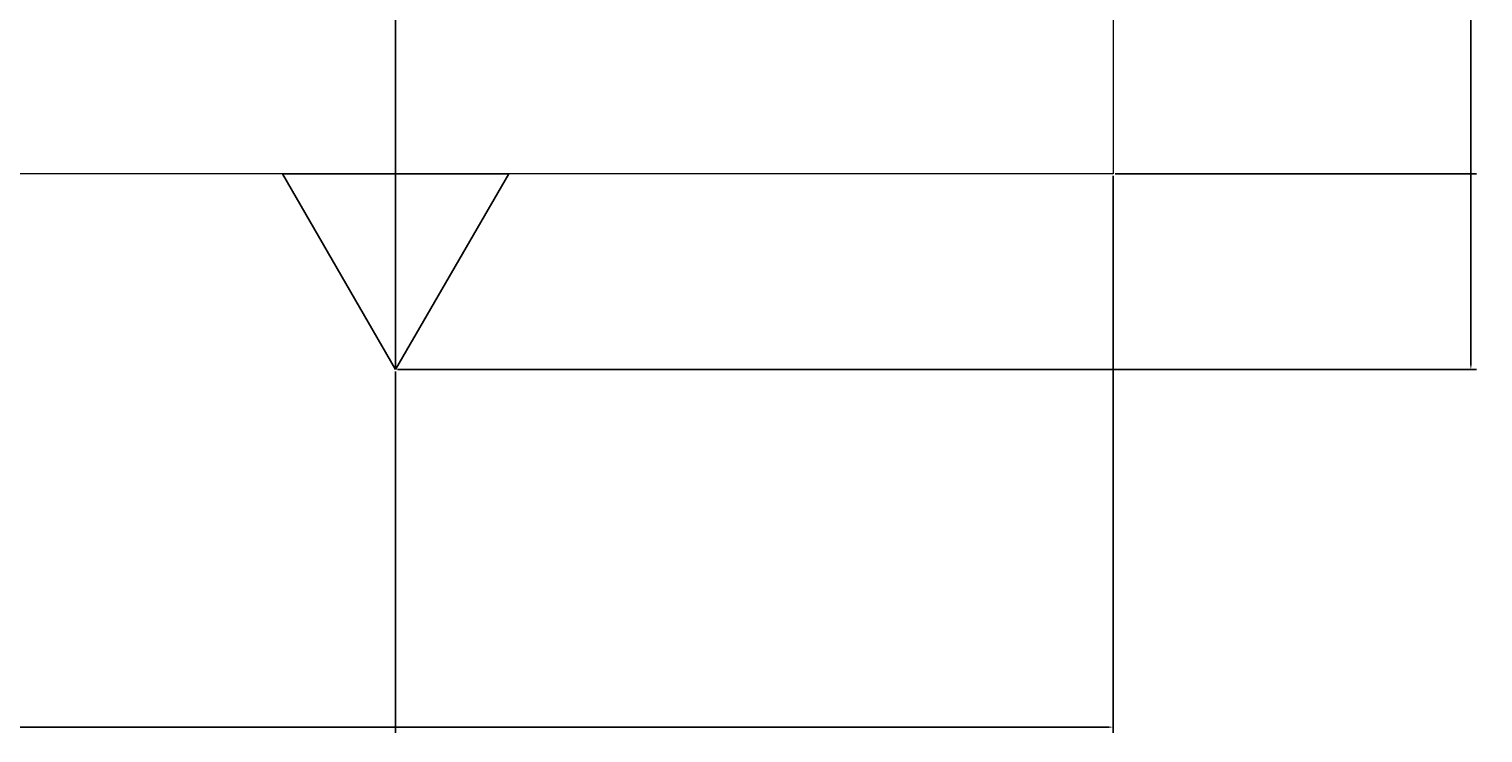
# Model space of a CAD drawing. Units: inches. Extents: x 412 to 584, y 208 to 437.
# Tile 9 of 28: x 539 to 584, y 208 to 230. Entities that reach past the tile are written whole.
import ezdxf

# ---------------------------------------------------------------- set-up
doc = ezdxf.new("R2010")
doc.units = ezdxf.units.IN
doc.header["$MEASUREMENT"] = 0
for name, color, linetype, lineweight in [('A-ANNO-DIMS', 2, 'Continuous', 18), ('E-ENCL', 8, 'Continuous', 18), ('E-POWR-EQPM', 3, 'Continuous', 25)]:
    doc.layers.add(name, color=color, linetype=linetype, lineweight=lineweight)
doc.styles.get("Standard").update_dxf_attribs({"font": 'arial.ttf'})
doc.dimstyles.get("Standard").update_dxf_attribs({"dimtxt": 0.18, "dimasz": 0.18, "dimexe": 0.18, "dimexo": 0.0625, "dimgap": 0.09, "dimtad": 0, "dimtih": 1, "dimtoh": 1, "dimdec": 4, "dimzin": 0, "dimdsep": 46, "dimtxsty": 'Standard', "dimcen": 0.09, "dimadec": 0, "dimazin": 0, "dimtfac": 1, "dimtdec": 4, "dimtofl": 0, "dimtmove": 0, "dimatfit": 3, "dimfxl": 1, "dimtolj": 1, "dimtzin": 0, "dimarcsym": 0})

# ---------------------------------------------------------------- blocks, each defined once
blk = doc.blocks.new('*U3')
blk.add_line((-0.212, 0.212), (0.212, -0.212))
blk = doc.blocks.new('*U4')
at = {"color": 0, "linetype": 'ByBlock', "lineweight": -2, "transparency": 16777216}
for p, rotation in [((224.254, 56.203), 180), ((224.677, 56.203), 89.99999999999999), ((224.254, 55.78), 269.9999999999999)]:
    blk.add_blockref('*U3', p, dxfattribs=dict(at, rotation=rotation))
blk.add_blockref('*U3', (224.677, 55.78), dxfattribs=at)
blk = doc.blocks.new('*U7')
blk.add_line((-0.288, 0.288), (0.288, -0.288))
blk = doc.blocks.new('*U8')
at = {"color": 0, "linetype": 'ByBlock', "lineweight": -2, "transparency": 16777216}
for p, rotation in [((224.177, 56.28), 180), ((224.754, 56.28), 90), ((224.177, 55.703), 269.9999999999999)]:
    blk.add_blockref('*U7', p, dxfattribs=dict(at, rotation=rotation))
blk.add_blockref('*U7', (224.754, 55.703), dxfattribs=at)
blk = doc.blocks.new('MCCB-800A')
for q in [(1.94, 18.628), (3.361, 0)]:
    blk.add_line((3.361, 14.893), q)
blk.add_lwpolyline([(0, 20.016), (6.722, 20.016), (6.722, 12.209), (0, 12.209)], close=True)
blk.add_circle((3.361, 14.5), 0.393)
for name in ['*U8', '*U4']:
    blk.add_blockref(name, (-221.104, -36.809))
blk = doc.blocks.new('*D13')
at = {"layer": 'A-ANNO-DIMS', "color": 0, "lineweight": -2, "transparency": 16777216}
for p, q in [((423.556, 225.526), (423.556, 208.233)), ((572.394, 225.526), (572.394, 208.233)), ((423.736, 208.413), (497.52, 208.413)), ((572.214, 208.413), (498.43, 208.413))]:
    blk.add_line(p, q, dxfattribs=at)
at = {"layer": 'A-ANNO-DIMS', "color": 0, "transparency": 16777216}
for points in [[(423.736, 208.443), (423.736, 208.383), (423.556, 208.413)], [(572.214, 208.443), (572.214, 208.383), (572.394, 208.413)]]:
    blk.add_solid(points, dxfattribs=at)
at = {"layer": 'Defpoints', "color": 0, "transparency": 16777216}
for p in [(423.556, 225.588), (572.394, 225.588), (572.394, 208.413)]:
    blk.add_point(p, dxfattribs=at)
at = {"layer": 'A-ANNO-DIMS', "color": 0, "transparency": 16777216, "insert": (497.975, 208.413), "char_height": 0.18, "attachment_point": 5}
blk.add_mtext('\\A1;148.84', dxfattribs=at)
blk = doc.blocks.new('*D16')
at = {"layer": 'A-ANNO-DIMS', "color": 0, "lineweight": -2, "transparency": 16777216}
for p, q in [((499.288, 219.47), (499.288, 208.233)), ((550.135, 219.451), (550.135, 208.233)), ((499.468, 208.413), (524.317, 208.413)), ((549.955, 208.413), (525.106, 208.413))]:
    blk.add_line(p, q, dxfattribs=at)
at = {"layer": 'A-ANNO-DIMS', "color": 0, "transparency": 16777216}
for points in [[(499.468, 208.443), (499.468, 208.383), (499.288, 208.413)], [(549.955, 208.443), (549.955, 208.383), (550.135, 208.413)]]:
    blk.add_solid(points, dxfattribs=at)
at = {"layer": 'Defpoints', "color": 0, "transparency": 16777216}
for p in [(499.288, 219.533), (550.135, 219.513), (550.135, 208.413)]:
    blk.add_point(p, dxfattribs=at)
at = {"layer": 'A-ANNO-DIMS', "color": 0, "transparency": 16777216, "insert": (524.711, 208.413), "char_height": 0.18, "attachment_point": 5}
blk.add_mtext('\\A1;50.85', dxfattribs=at)
blk = doc.blocks.new('*D17')
at = {"layer": 'A-ANNO-DIMS', "color": 0, "lineweight": -2, "transparency": 16777216}
for p, q in [((497.715, 426.185), (583.674, 426.185)), ((583.494, 426.005), (583.494, 323.031)), ((583.494, 219.693), (583.494, 322.667)), ((550.198, 219.513), (583.674, 219.513))]:
    blk.add_line(p, q, dxfattribs=at)
at = {"layer": 'A-ANNO-DIMS', "color": 0, "transparency": 16777216}
for points in [[(583.464, 426.005), (583.524, 426.005), (583.494, 426.185)], [(583.464, 219.693), (583.524, 219.693), (583.494, 219.513)]]:
    blk.add_solid(points, dxfattribs=at)
at = {"layer": 'Defpoints', "color": 0, "transparency": 16777216}
for p in [(497.652, 426.185), (550.135, 219.513), (583.494, 219.513)]:
    blk.add_point(p, dxfattribs=at)
at = {"layer": 'A-ANNO-DIMS', "color": 0, "transparency": 16777216, "insert": (583.494, 322.849), "char_height": 0.18, "attachment_point": 5}
blk.add_mtext('\\A1;206.67', dxfattribs=at)
blk = doc.blocks.new('*D18')
at = {"layer": 'A-ANNO-DIMS', "color": 0, "lineweight": -2, "transparency": 16777216}
for p, q in [((572.456, 309.377), (583.674, 309.377)), ((583.494, 309.197), (583.494, 267.665)), ((583.494, 225.768), (583.494, 267.301)), ((572.456, 225.588), (583.674, 225.588))]:
    blk.add_line(p, q, dxfattribs=at)
at = {"layer": 'A-ANNO-DIMS', "color": 0, "transparency": 16777216}
for points in [[(583.464, 309.197), (583.524, 309.197), (583.494, 309.377)], [(583.464, 225.768), (583.524, 225.768), (583.494, 225.588)]]:
    blk.add_solid(points, dxfattribs=at)
at = {"layer": 'Defpoints', "color": 0, "transparency": 16777216}
for p in [(572.394, 309.377), (572.394, 225.588), (583.494, 225.588)]:
    blk.add_point(p, dxfattribs=at)
at = {"layer": 'A-ANNO-DIMS', "color": 0, "transparency": 16777216, "insert": (583.494, 267.483), "char_height": 0.18, "attachment_point": 5}
blk.add_mtext('\\A1;83.79', dxfattribs=at)
blk = doc.blocks.new('*D19')
at = {"layer": 'A-ANNO-DIMS', "color": 0, "lineweight": -2, "transparency": 16777216}
for p, q in [((555.858, 256.573), (583.674, 256.573)), ((583.494, 256.393), (583.494, 241.263)), ((583.494, 225.768), (583.494, 240.899)), ((572.456, 225.588), (583.674, 225.588))]:
    blk.add_line(p, q, dxfattribs=at)
at = {"layer": 'A-ANNO-DIMS', "color": 0, "transparency": 16777216}
for points in [[(583.464, 256.393), (583.524, 256.393), (583.494, 256.573)], [(583.464, 225.768), (583.524, 225.768), (583.494, 225.588)]]:
    blk.add_solid(points, dxfattribs=at)
at = {"layer": 'Defpoints', "color": 0, "transparency": 16777216}
for p in [(555.796, 256.573), (572.394, 225.588), (583.494, 225.588)]:
    blk.add_point(p, dxfattribs=at)
at = {"layer": 'A-ANNO-DIMS', "color": 0, "transparency": 16777216, "insert": (583.494, 241.081), "char_height": 0.18, "attachment_point": 5}
blk.add_mtext('\\A1;30.985', dxfattribs=at)

msp = doc.modelspace()

# ---------------------------------------------------------------- linework, layer by layer
at = {"layer": 'E-ENCL'}
msp.add_lwpolyline([(423.5562, 309.3773), (572.3937, 309.3773), (572.3937, 225.5881), (423.5562, 225.5881)], close=True, dxfattribs=at)
at = {"layer": 'E-POWR-EQPM'}
msp.add_line((550.1351, 219.5133), (550.1351, 225.5881), dxfattribs=at)
msp.add_lwpolyline([(550.1351, 219.5133), (553.6424, 225.5881), (546.6278, 225.5881)], close=True, dxfattribs=at)

# ---------------------------------------------------------------- block references
msp.add_blockref('MCCB-800A', (546.774, 225.588), dxfattribs=at)

# ---------------------------------------------------------------- dimensions: what is measured, and where the dimension line sits
at = {"layer": 'A-ANNO-DIMS'}
for base, p1, p2, override, picture, middle in [((583.4937, 219.5133), (497.6523, 426.1847), (550.1351, 219.5133), {"dimdec": 2, "dimlfac": 1, "dimrnd": 0, "dimzin": 0, "dimdsep": 46, "dimlunit": 2}, '*D17', (583.4937, 322.849)), ((583.4937, 225.5881), (572.3937, 309.3773), (572.3937, 225.5881), {"dimdec": 2, "dimlfac": 1, "dimrnd": 0, "dimzin": 0, "dimdsep": 46, "dimlunit": 2}, '*D18', (583.4937, 267.4827)), ((583.4937, 225.5881), (555.7959, 256.5729), (572.3937, 225.5881), {"dimdec": 3, "dimlfac": 1, "dimrnd": 0, "dimzin": 0, "dimdsep": 46, "dimlunit": 2}, '*D19', (583.4937, 241.0805))]:
    dim = msp.add_linear_dim(base=base, p1=p1, p2=p2, angle=90, dimstyle='Standard', override=override, dxfattribs=at)
    dim.commit()
    dim.dimension.update_dxf_attribs({"geometry": picture, "text_midpoint": middle})
for base, p1, p2, picture, middle in [((572.3937, 208.4133), (423.5562, 225.5881), (572.3937, 225.5881), '*D13', (497.975, 208.4133)), ((550.1351, 208.4133), (499.2878, 219.5329), (550.1351, 219.5133), '*D16', (524.7115, 208.4133))]:
    dim = msp.add_linear_dim(base=base, p1=p1, p2=p2, dimstyle='Standard', override={"dimdec": 2, "dimlfac": 1, "dimrnd": 0, "dimzin": 0, "dimdsep": 46, "dimlunit": 2}, dxfattribs=at)
    dim.commit()
    dim.dimension.update_dxf_attribs({"geometry": picture, "text_midpoint": middle})

doc.saveas('drawing.dxf')
